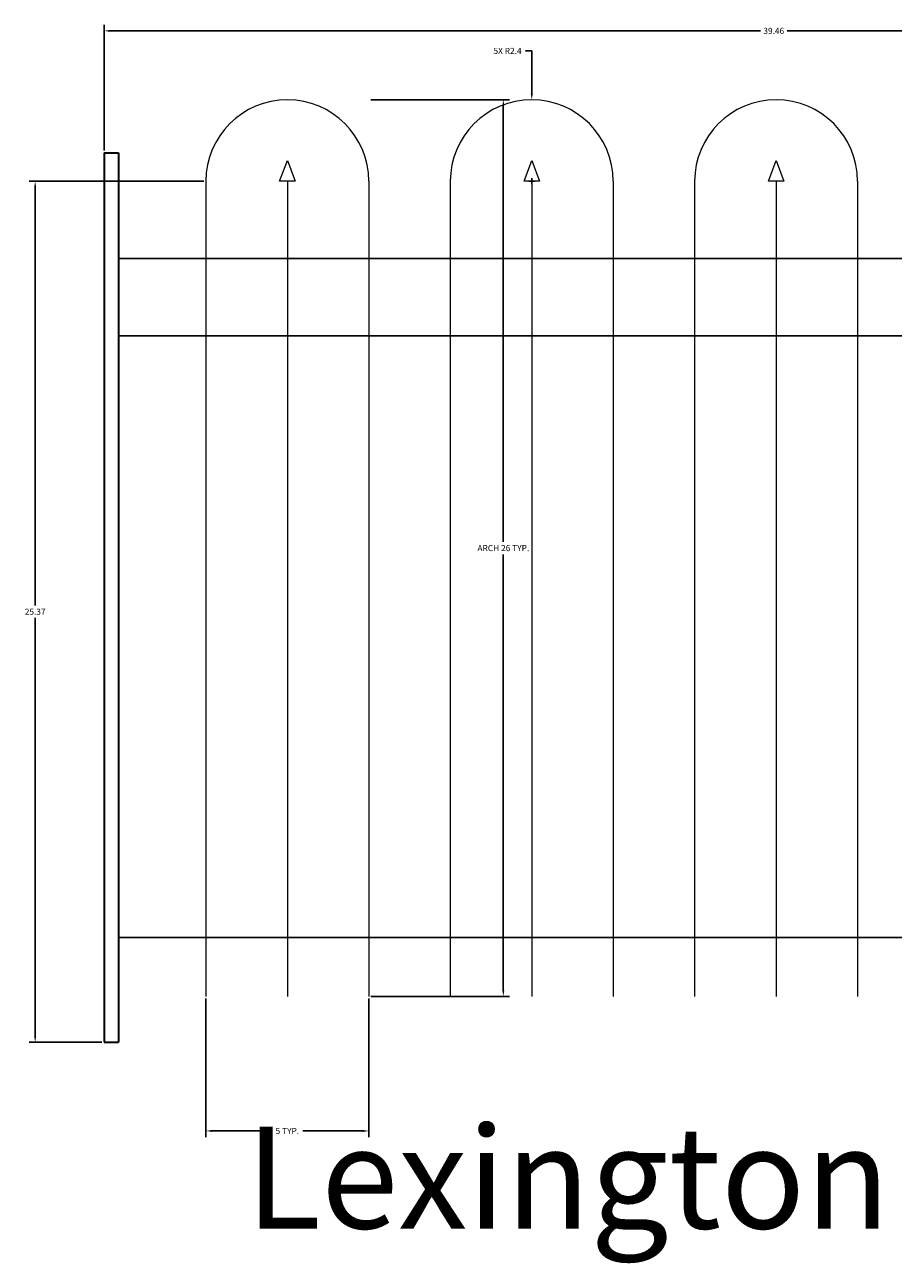
# Model space of a CAD drawing. Units: inches. Extents: x 756 to 915, y 488 to 695.
# Tile 11 of 25: x 768 to 794, y 587 to 624. Entities that reach past the tile are written whole.
import ezdxf

# ---------------------------------------------------------------- set-up
doc = ezdxf.new("R2010")
doc.units = ezdxf.units.IN
doc.header["$MEASUREMENT"] = 0
for name, color, linetype, lineweight in [('L-ANNO-TEXT', 7, 'Continuous', 25), ('L-FENC-PCKT', 7, 'Continuous', 18), ('L-FENC-POST', 7, 'Continuous', 35), ('L-FENC-RAIL', 7, 'Continuous', 25), ('M-DIMS', 2, 'Continuous', 18)]:
    doc.layers.add(name, color=color, linetype=linetype, lineweight=lineweight)
doc.styles.get("Standard").update_dxf_attribs({"font": 'arial.ttf'})
doc.dimstyles.get("Standard").update_dxf_attribs({"dimtxt": 0.18, "dimasz": 0.18, "dimexe": 0.18, "dimexo": 0.0625, "dimgap": 0.09, "dimtad": 0, "dimtih": 1, "dimtoh": 1, "dimdec": 0, "dimzin": 0, "dimdsep": 46, "dimlunit": 3, "dimtxsty": 'Standard', "dimcen": 0.09, "dimadec": 0, "dimazin": 0, "dimtfac": 1, "dimtdec": 0, "dimtofl": 0, "dimtmove": 0, "dimatfit": 3, "dimfxl": 1, "dimtolj": 1, "dimtzin": 0, "dimarcsym": 0})

# ---------------------------------------------------------------- blocks, each defined once
blk = doc.blocks.new('FENCE-POST-LEFT')
for p, q in [((0, 26.207), (0, 0)), ((0, 26.207), (0.426, 26.207)), ((0.426, 26.207), (0.426, 0)), ((0.426, 26.207), (0.426, 0)), ((0, 0), (0.426, 0))]:
    blk.add_line(p, q)
blk = doc.blocks.new('PICKET-ROUND-ARCH')
for p, q in [((0, 24.019), (0, 0)), ((4.8, 24.019), (4.8, 0))]:
    blk.add_line(p, q)
blk.add_arc((2.4, 24.019), 2.4, 0, 180)
blk = doc.blocks.new('PICKET-SPEAR-ARCH-INFILL')
blk.add_line((0.227, 24.019), (0.227, 0))
blk.add_lwpolyline([(0.227, 24.019), (0, 24.019), (0.227, 24.631), (0.455, 24.019)], close=True)
blk = doc.blocks.new('*D11')
at = {"layer": 'Defpoints', "color": 0, "transparency": 16777216}
for p in [(778.57, 621.653), (782.533, 621.653), (778.57, 595.234)]:
    blk.add_point(p, dxfattribs=at)
at = {"layer": 'M-DIMS', "color": 0, "lineweight": -2, "transparency": 16777216}
for p, q in [((778.633, 621.653), (782.713, 621.653)), ((782.533, 621.473), (782.533, 608.627)), ((782.533, 595.414), (782.533, 608.26)), ((778.633, 595.234), (782.713, 595.234))]:
    blk.add_line(p, q, dxfattribs=at)
at = {"layer": 'M-DIMS', "color": 0, "transparency": 16777216}
for points in [[(782.503, 621.473), (782.563, 621.473), (782.533, 621.653)], [(782.503, 595.414), (782.563, 595.414), (782.533, 595.234)]]:
    blk.add_solid(points, dxfattribs=at)
at = {"layer": 'M-DIMS', "color": 0, "transparency": 16777216, "insert": (782.533, 608.444), "char_height": 0.18, "attachment_point": 5}
blk.add_mtext('\\A1;ARCH 26 TYP.', dxfattribs=at)
blk = doc.blocks.new('*D12')
at = {"layer": 'Defpoints', "color": 0, "transparency": 16777216}
for p in [(773.77, 595.234), (778.57, 595.234), (778.57, 591.271)]:
    blk.add_point(p, dxfattribs=at)
at = {"layer": 'M-DIMS', "color": 0, "lineweight": -2, "transparency": 16777216}
for p, q in [((773.77, 595.172), (773.77, 591.091)), ((778.57, 595.172), (778.57, 591.091)), ((773.95, 591.271), (775.712, 591.271)), ((778.39, 591.271), (776.629, 591.271))]:
    blk.add_line(p, q, dxfattribs=at)
at = {"layer": 'M-DIMS', "color": 0, "transparency": 16777216}
for points in [[(773.95, 591.301), (773.95, 591.241), (773.77, 591.271)], [(778.39, 591.301), (778.39, 591.241), (778.57, 591.271)]]:
    blk.add_solid(points, dxfattribs=at)
at = {"layer": 'M-DIMS', "color": 0, "transparency": 16777216, "insert": (776.17, 591.271), "char_height": 0.18, "attachment_point": 5}
blk.add_mtext('\\A1;5 TYP.', dxfattribs=at)
blk = doc.blocks.new('*D49')
at = {"layer": 'Defpoints', "color": 0, "transparency": 16777216}
for p in [(810.23, 623.683), (770.771, 620.092), (810.23, 620.092)]:
    blk.add_point(p, dxfattribs=at)
at = {"layer": 'M-DIMS', "color": 0, "lineweight": -2, "transparency": 16777216}
for p, q in [((770.771, 620.154), (770.771, 623.863)), ((770.951, 623.683), (790.107, 623.683)), ((810.05, 623.683), (790.894, 623.683)), ((810.23, 620.154), (810.23, 623.863))]:
    blk.add_line(p, q, dxfattribs=at)
at = {"layer": 'M-DIMS', "color": 0, "transparency": 16777216}
for points in [[(770.951, 623.713), (770.951, 623.653), (770.771, 623.683)], [(810.05, 623.713), (810.05, 623.653), (810.23, 623.683)]]:
    blk.add_solid(points, dxfattribs=at)
at = {"layer": 'M-DIMS', "color": 0, "transparency": 16777216, "insert": (790.5, 623.683), "char_height": 0.18, "attachment_point": 5}
blk.add_mtext('\\A1;39.46', dxfattribs=at)
blk = doc.blocks.new('*D51')
at = {"layer": 'Defpoints', "color": 0, "transparency": 16777216}
for p in [(768.741, 619.253), (773.77, 619.253), (770.771, 593.885)]:
    blk.add_point(p, dxfattribs=at)
at = {"layer": 'M-DIMS', "color": 0, "lineweight": -2, "transparency": 16777216}
for p, q in [((773.708, 619.253), (768.561, 619.253)), ((768.741, 619.073), (768.741, 606.751)), ((768.741, 594.065), (768.741, 606.387)), ((770.709, 593.885), (768.561, 593.885))]:
    blk.add_line(p, q, dxfattribs=at)
at = {"layer": 'M-DIMS', "color": 0, "transparency": 16777216}
for points in [[(768.711, 619.073), (768.771, 619.073), (768.741, 619.253)], [(768.711, 594.065), (768.771, 594.065), (768.741, 593.885)]]:
    blk.add_solid(points, dxfattribs=at)
at = {"layer": 'M-DIMS', "color": 0, "transparency": 16777216, "insert": (768.741, 606.569), "char_height": 0.18, "attachment_point": 5}
blk.add_mtext('\\A1;25.37', dxfattribs=at)
blk = doc.blocks.new('*D79')
at = {"layer": 'Defpoints', "color": 0, "transparency": 16777216}
for p in [(783.37, 621.653), (783.37, 619.253)]:
    blk.add_point(p, dxfattribs=at)
at = {"layer": 'M-DIMS', "color": 0, "lineweight": -2, "transparency": 16777216}
for p, q in [((783.19, 623.093), (783.37, 623.093)), ((783.37, 623.093), (783.37, 621.833)), ((783.28, 619.253), (783.46, 619.253)), ((783.37, 619.163), (783.37, 619.343))]:
    blk.add_line(p, q, dxfattribs=at)
at = {"layer": 'M-DIMS', "color": 0, "transparency": 16777216}
blk.add_solid([(783.4, 621.833), (783.34, 621.833), (783.37, 621.653)], dxfattribs=at)
at = {"layer": 'M-DIMS', "color": 0, "transparency": 16777216, "insert": (782.657, 623.093), "char_height": 0.18, "attachment_point": 5}
blk.add_mtext('\\A1;5X R2.4', dxfattribs=at)

msp = doc.modelspace()

# ---------------------------------------------------------------- linework, layer by layer
at = {"layer": 'L-FENC-RAIL'}
for p, q in [((771.198, 616.9765), (809.8029, 616.9765)), ((771.198, 614.7001), (809.8029, 614.7001)), ((771.198, 596.9663), (809.8029, 596.9663))]:
    msp.add_line(p, q, dxfattribs=at)

# ---------------------------------------------------------------- block references
at = {"layer": 'L-FENC-PCKT'}
for name, p in [('PICKET-ROUND-ARCH', (773.77, 595.234)), ('PICKET-ROUND-ARCH', (780.9697, 595.234)), ('PICKET-ROUND-ARCH', (788.1695, 595.234)), ('PICKET-SPEAR-ARCH-INFILL', (775.943, 595.234)), ('PICKET-SPEAR-ARCH-INFILL', (783.1427, 595.234)), ('PICKET-SPEAR-ARCH-INFILL', (790.3425, 595.234))]:
    msp.add_blockref(name, p, dxfattribs=at)
at = {"layer": 'L-FENC-POST'}
msp.add_blockref('FENCE-POST-LEFT', (770.7717, 593.8847), dxfattribs=at)

# ---------------------------------------------------------------- texts
at = {"layer": 'L-ANNO-TEXT'}
msp.add_text('Lexington', height=3, dxfattribs=at).set_placement((774.9436, 588.3968))

# ---------------------------------------------------------------- dimensions: what is measured, and where the dimension line sits
at = {"layer": 'M-DIMS'}
dim = msp.add_linear_dim(base=(810.2295, 623.6829), p1=(770.7714, 620.0915), p2=(810.2295, 620.0915), dimstyle='Standard', override={"dimdec": 2, "dimlfac": 1, "dimrnd": 0, "dimzin": 0, "dimdsep": 46, "dimlunit": 2}, dxfattribs=at)
dim.commit()
dim.dimension.update_dxf_attribs({"geometry": '*D49', "text_midpoint": (790.5004, 623.6829)})
dim = msp.add_radius_dim(center=(783.3701, 619.2529), mpoint=(783.37, 621.6529), text='5X <>', dimstyle='Standard', override={"dimdec": 1, "dimlfac": 1, "dimrnd": 0, "dimzin": 0, "dimdsep": 46, "dimlunit": 2}, dxfattribs=at)
dim.commit()
dim.dimension.update_dxf_attribs({"geometry": '*D79', "text_midpoint": (782.6569, 623.0928), "dimtype": 164})
dim = msp.add_linear_dim(base=(782.5331, 621.6529), p1=(778.5703, 595.2343), p2=(778.5703, 621.6529), angle=90, text='ARCH <> TYP.', dimstyle='Standard', override={"dimdec": 0, "dimlfac": 1, "dimrnd": 0, "dimzin": 0, "dimdsep": 46, "dimlunit": 2}, dxfattribs=at)
dim.commit()
dim.dimension.update_dxf_attribs({"geometry": '*D11', "text_midpoint": (782.5331, 608.4436)})
dim = msp.add_linear_dim(base=(768.7414, 619.2529), p1=(770.7714, 593.8847), p2=(773.7705, 619.2529), angle=90, dimstyle='Standard', override={"dimdec": 2, "dimlfac": 1, "dimrnd": 0, "dimzin": 0, "dimdsep": 46, "dimlunit": 2}, dxfattribs=at)
dim.commit()
dim.dimension.update_dxf_attribs({"geometry": '*D51', "text_midpoint": (768.7414, 606.5688)})
dim = msp.add_linear_dim(base=(778.5703, 591.2715), p1=(773.7705, 595.2343), p2=(778.5703, 595.2343), text='<> TYP.', dimstyle='Standard', override={"dimdec": 0, "dimlfac": 1, "dimrnd": 0, "dimzin": 0, "dimdsep": 46, "dimlunit": 2}, dxfattribs=at)
dim.commit()
dim.dimension.update_dxf_attribs({"geometry": '*D12', "text_midpoint": (776.1704, 591.2715)})

doc.saveas('drawing.dxf')
